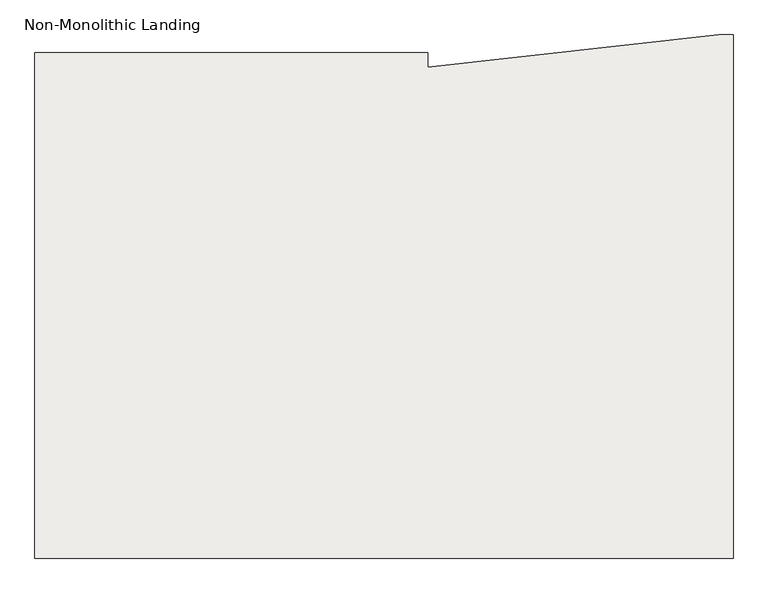
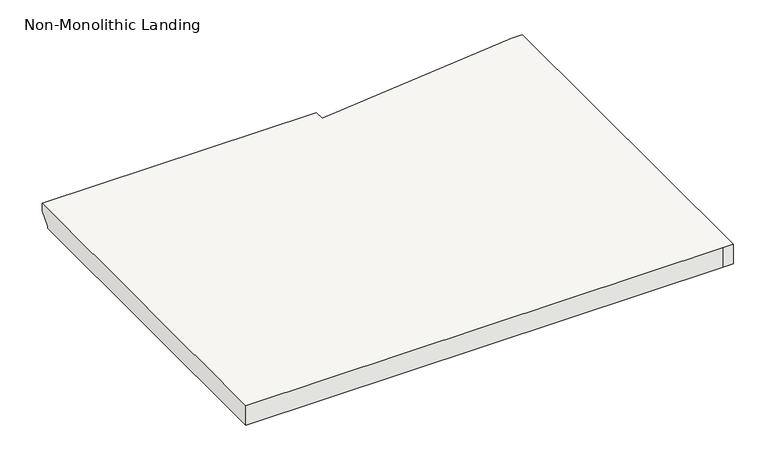
"""IFC4 building model written with IfcOpenShell, lengths in millimetres: slab geometry, Non-Monolithic Landing."""

from ifc_helpers import new_model, si_unit, origin, place, context, project, spatial, faceted_brep, source, transform, mapped, element, save


def non_monolithic_landing_7f41dad4(model_context):
    return source(origin(), model_context, "Body", "Brep", [
        faceted_brep([(-10581.8342448, -2032.7993654, 2317.75), (-10581.8342448, -2032.7993654, 2336.8), (-10581.8342448, -2058.1993654, 2336.8), (-10581.8342448, -2058.1993654, 2292.35), (-11268.1522729, -2032.7993654, 2317.75), (-11268.1522729, -2032.7993654, 2336.8), (-11268.1522729, -2058.1993654, 2292.35), (-11268.1522729, -2916.0844117, 2336.8), (-10074.3522729, -2916.0844117, 2336.8), (-10048.9522729, -2916.0844117, 2336.8), (-10048.9522729, -2001.6844117, 2336.8), (-10074.3522729, -2001.6844117, 2336.8), (-11268.1522729, -2058.1993654, 2286.0), (-10581.8342448, -2058.1993654, 2286.0), (-10074.3522729, -2001.6844117, 2286.0), (-10048.9522729, -2001.6844117, 2286.0), (-10048.9522729, -2916.0844117, 2286.0), (-10074.3522729, -2916.0844117, 2286.0), (-11268.1522729, -2916.0844117, 2286.0)], [[[0, 1, 2, 3]], [[4, 5, 1, 0]], [[6, 4, 0, 3]], [[7, 8, 9, 10, 11, 2, 1, 5]], [[12, 13, 14, 15, 16, 17, 18]], [[13, 12, 6, 3]], [[7, 5, 4, 6, 12, 18]], [[8, 7, 18, 17]], [[9, 8, 17, 16]], [[10, 9, 16, 15]], [[11, 10, 15, 14]], [[2, 11, 14, 13, 3]]]),
    ])


if __name__ == "__main__":
    model = new_model("IFC4")
    model_context = context("Model", 3, world=origin())
    ifc_project = project(units=[si_unit("LENGTHUNIT", "METRE", prefix="MILLI")], contexts=[model_context])
    site = spatial("IfcSite", under=ifc_project)
    building = spatial("IfcBuilding", under=site)
    placement = place(None, origin())
    non_monolithic_landing_shape = non_monolithic_landing_7f41dad4(model_context)
    element("IfcSlab", 1, ObjectType="Non-Monolithic Landing", at=placement, inside=building, context=model_context, shape_type="MappedRepresentation", body=[
        mapped(non_monolithic_landing_shape, transform((0.0, 0.0, 0.0), x_axis=(1.0, 0.0, 0.0), y_axis=(0.0, 1.0, 0.0), z_axis=(0.0, 0.0, 1.0))),
    ])
    save(model, "model.ifc")
